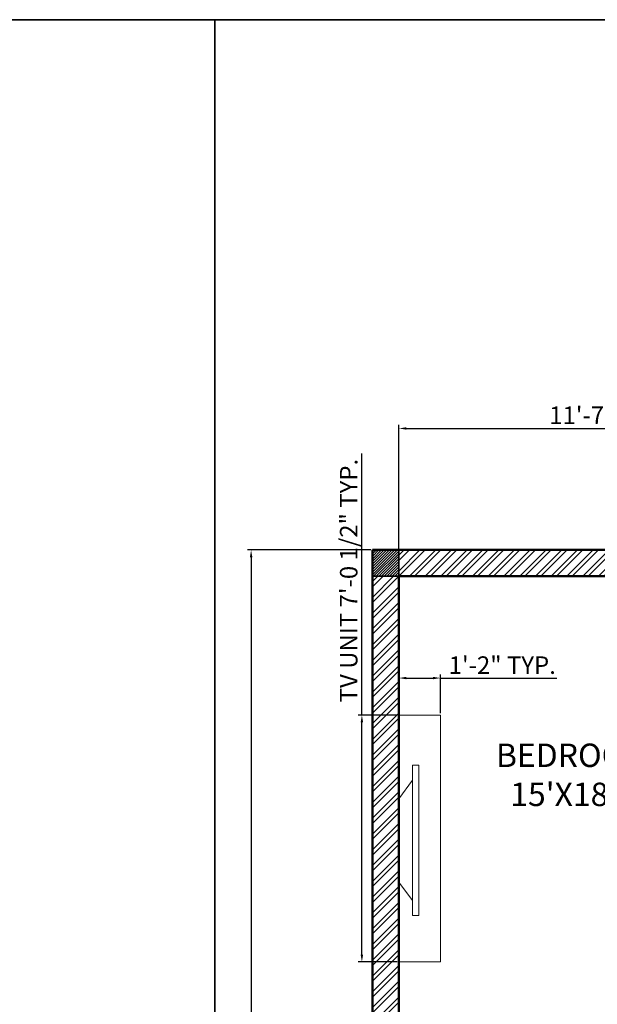
# Model space of a CAD drawing. Units: millimetres. Extents: x 20768 to 23556, y 50760 to 52704.
# Tile 26 of 36: x 21205 to 21403, y 52368 to 52704. Entities that reach past the tile are written whole.
import ezdxf

# ---------------------------------------------------------------- set-up
doc = ezdxf.new("R2010")
doc.units = ezdxf.units.MM
for name, color, linetype, lineweight in [('A-ANNO-TTLB', 7, 'Continuous', 35), ('A-AREA-IDEN', 40, 'Continuous', 18), ('A-FURN', 8, 'Continuous', 18), ('A-WALL', 7, 'Continuous', 50), ('A-WALL-PATT', 8, 'Continuous', 13), ('S-ANNO-DIMS', 2, 'Continuous', 18), ('S-COLS', 20, 'Continuous', 35)]:
    doc.layers.add(name, color=color, linetype=linetype, lineweight=lineweight)
doc.styles.get("Standard").update_dxf_attribs({"font": 'arial.ttf'})
doc.dimstyles.new('ISO-25', dxfattribs={"dimtxt": 6, "dimasz": 2.5, "dimexe": 1.25, "dimexo": 0.625, "dimtad": 1, "dimdec": 0, "dimlunit": 3, "dimtxsty": 'Standard', "dimcen": 2.5, "dimadec": 0, "dimazin": 0, "dimtfac": 1, "dimtdec": 0, "dimtmove": 0, "dimatfit": 3, "dimfxl": 1, "dimarcsym": 0})
pattern_1 = [(45, (-37.4434, 0), (-2.69407684, 2.69407684), []), (45, (-35.6473, 0), (-2.69407684, 2.69407684), [])]

# ---------------------------------------------------------------- blocks, each defined once
blk = doc.blocks.new('tv')
for p, q in [((20989.25, 52437.95), (20993.93, 52444.3)), ((20989.25, 52409.51), (20993.93, 52403.15))]:
    blk.add_line(p, q)
for points in [[(20989.25, 52466.51), (21003.46, 52466.51), (21003.46, 52382.21), (20989.25, 52382.21)], [(20993.93, 52449.42), (20996.05, 52449.42), (20996.05, 52398.03), (20993.93, 52398.03)]]:
    blk.add_lwpolyline(points, close=True)
blk = doc.blocks.new('*D183')
at = {"layer": 'Defpoints', "color": 0, "transparency": 16777216}
for p in [(21322.1, 52466.51), (21334.74, 52466.51), (21334.74, 52382.21)]:
    blk.add_point(p, dxfattribs=at)
at = {"layer": 'S-ANNO-DIMS', "color": 0, "lineweight": -2, "transparency": 16777216}
for p, q in [((21322.1, 52466.51), (21322.1, 52555.89)), ((21334.12, 52466.51), (21320.85, 52466.51)), ((21322.1, 52384.71), (21322.1, 52464.01)), ((21334.12, 52382.21), (21320.85, 52382.21))]:
    blk.add_line(p, q, dxfattribs=at)
at = {"layer": 'S-ANNO-DIMS', "color": 0, "transparency": 16777216}
for points in [[(21321.68, 52464.01), (21322.51, 52464.01), (21322.1, 52466.51)], [(21321.68, 52384.71), (21322.51, 52384.71), (21322.1, 52382.21)]]:
    blk.add_solid(points, dxfattribs=at)
at = {"layer": 'S-ANNO-DIMS', "color": 0, "transparency": 16777216, "insert": (21318.37, 52512.45), "char_height": 6, "attachment_point": 5, "rotation": 90}
blk.add_mtext('TV UNIT 7\'-0 1/2" TYP.', dxfattribs=at)
blk = doc.blocks.new('*D184')
at = {"layer": 'Defpoints', "color": 0, "transparency": 16777216}
for p in [(21348.95, 52479.16), (21334.74, 52466.51), (21348.95, 52466.51)]:
    blk.add_point(p, dxfattribs=at)
at = {"layer": 'S-ANNO-DIMS', "color": 0, "lineweight": -2, "transparency": 16777216}
for p, q in [((21334.74, 52467.14), (21334.74, 52480.41)), ((21348.95, 52467.14), (21348.95, 52480.41)), ((21337.24, 52479.16), (21346.45, 52479.16)), ((21348.95, 52479.16), (21388.71, 52479.16))]:
    blk.add_line(p, q, dxfattribs=at)
at = {"layer": 'S-ANNO-DIMS', "color": 0, "transparency": 16777216}
for points in [[(21337.24, 52479.57), (21337.24, 52478.74), (21334.74, 52479.16)], [(21346.45, 52479.57), (21346.45, 52478.74), (21348.95, 52479.16)]]:
    blk.add_solid(points, dxfattribs=at)
at = {"layer": 'S-ANNO-DIMS', "color": 0, "transparency": 16777216, "insert": (21370.08, 52482.79), "char_height": 6, "attachment_point": 5}
blk.add_mtext('1\'-2" TYP.', dxfattribs=at)
blk = doc.blocks.new('*D211')
at = {"layer": 'Defpoints', "color": 0, "transparency": 16777216}
for p in [(21325.74, 52522.9), (21284.24, 51829.9), (21325.74, 51829.9)]:
    blk.add_point(p, dxfattribs=at)
at = {"layer": 'S-ANNO-DIMS', "color": 0, "lineweight": -2, "transparency": 16777216}
for p, q in [((21325.12, 52522.9), (21282.99, 52522.9)), ((21284.24, 52520.4), (21284.24, 51832.4)), ((21325.12, 51829.9), (21282.99, 51829.9))]:
    blk.add_line(p, q, dxfattribs=at)
at = {"layer": 'S-ANNO-DIMS', "color": 0, "transparency": 16777216}
for points in [[(21283.82, 52520.4), (21284.66, 52520.4), (21284.24, 52522.9)], [(21283.82, 51832.4), (21284.66, 51832.4), (21284.24, 51829.9)]]:
    blk.add_solid(points, dxfattribs=at)
at = {"layer": 'S-ANNO-DIMS', "color": 0, "transparency": 16777216, "insert": (21280.55, 52176.4), "char_height": 6, "attachment_point": 5, "rotation": 90}
blk.add_mtext('57\'-9"', dxfattribs=at)
blk = doc.blocks.new('*D215')
at = {"layer": 'Defpoints', "color": 0, "transparency": 16777216}
for p in [(21474.24, 52564.4), (21334.74, 52329.4), (21474.24, 52329.4)]:
    blk.add_point(p, dxfattribs=at)
at = {"layer": 'S-ANNO-DIMS', "color": 0, "lineweight": -2, "transparency": 16777216}
for p, q in [((21334.74, 52330.02), (21334.74, 52565.65)), ((21337.24, 52564.4), (21471.74, 52564.4)), ((21474.24, 52330.02), (21474.24, 52565.65))]:
    blk.add_line(p, q, dxfattribs=at)
at = {"layer": 'S-ANNO-DIMS', "color": 0, "transparency": 16777216}
for points in [[(21337.24, 52564.81), (21337.24, 52563.98), (21334.74, 52564.4)], [(21471.74, 52564.81), (21471.74, 52563.98), (21474.24, 52564.4)]]:
    blk.add_solid(points, dxfattribs=at)
at = {"layer": 'S-ANNO-DIMS', "color": 0, "transparency": 16777216, "insert": (21404.49, 52568.12), "char_height": 6, "attachment_point": 5}
blk.add_mtext('11\'-7 1/2"', dxfattribs=at)

msp = doc.modelspace()

# ---------------------------------------------------------------- hatches: boundary and pattern name
at = {"layer": 'A-WALL-PATT'}
h = msp.add_hatch(dxfattribs=at)
h.set_pattern_fill('ANSI31', color=256, scale=0.2)
h.set_pattern_definition([(45, (345.4904, 0), (-0.449012806, 0.449012806), [])])
h.paths.add_polyline_path([(21334.74, 52522.9), (21325.74, 52522.9), (21325.74, 52513.9), (21334.74, 52513.9)])
h = msp.add_hatch(dxfattribs=at)
h.set_pattern_fill('ANSI32', color=256, scale=0.4)
h.set_pattern_definition(pattern_1)
h.paths.add_polyline_path([(21550.74, 52522.9), (21334.74, 52522.9), (21334.74, 52513.9), (21550.74, 52513.9)])
h = msp.add_hatch(dxfattribs=at)
h.set_pattern_fill('ANSI32', color=256, scale=0.4)
h.set_pattern_definition(pattern_1)
h.paths.add_polyline_path([(21334.74, 52513.9), (21325.74, 52513.9), (21325.74, 52335.9), (21334.74, 52335.9)])

# ---------------------------------------------------------------- linework, layer by layer
at = {"layer": 'A-ANNO-TTLB'}
msp.add_line((21271.86, 52703.98), (21271.86, 51623.53), dxfattribs=at)
msp.add_lwpolyline([(20768.14, 52703.98), (23555.8, 52703.98), (23555.8, 51623.53), (20768.14, 51623.53)], close=True, dxfattribs=at)
at = {"layer": 'A-WALL'}
for p, q in [((21325.74, 52522.9), (21325.74, 51829.9)), ((21325.74, 52522.9), (21559.74, 52522.9)), ((21334.74, 52513.9), (21334.74, 51829.9)), ((21334.74, 52513.9), (21550.74, 52513.9))]:
    msp.add_line(p, q, dxfattribs=at)
at = {"layer": 'S-COLS'}
msp.add_lwpolyline([(21334.74, 52513.9), (21325.74, 52513.9), (21325.74, 52522.9), (21334.74, 52522.9)], close=True, dxfattribs=at)

# ---------------------------------------------------------------- block references
at = {"layer": 'A-FURN'}
msp.add_blockref('tv', (345.49, 0), dxfattribs=at)

# ---------------------------------------------------------------- texts
at = {"layer": 'A-AREA-IDEN', "insert": (21367.92, 52456.78), "char_height": 8, "attachment_point": 1}
msp.add_mtext_dynamic_manual_height_columns("BEDROOM\\P  15'X18'", width=49.9521, gutter_width=12.5, heights=[0], dxfattribs=at)

# ---------------------------------------------------------------- dimensions: what is measured, and where the dimension line sits
at = {"layer": 'S-ANNO-DIMS'}
dim = msp.add_linear_dim(base=(21474.24, 52564.4), p1=(21334.74, 52329.4), p2=(21474.24, 52329.4), dimstyle='ISO-25', override={"dimdec": 1, "dimlfac": 1, "dimrnd": 0, "dimzin": 1, "dimdsep": 46, "dimlunit": 4, "dimfrac": 2}, dxfattribs=at)
dim.commit()
dim.dimension.update_dxf_attribs({"geometry": '*D215', "text_midpoint": (21404.49, 52568.12)})
dim = msp.add_linear_dim(base=(21322.1, 52466.51), p1=(21334.74, 52382.21), p2=(21334.74, 52466.51), angle=90, text='TV UNIT <> TYP.', dimstyle='ISO-25', override={"dimdec": 1, "dimrnd": 0, "dimzin": 1, "dimlunit": 4, "dimfrac": 2}, dxfattribs=at)
dim.commit()
dim.dimension.update_dxf_attribs({"geometry": '*D183', "text_midpoint": (21318.37, 52512.45)})
dim = msp.add_linear_dim(base=(21284.24, 51829.9), p1=(21325.74, 52522.9), p2=(21325.74, 51829.9), angle=90, dimstyle='ISO-25', override={"dimdec": 1, "dimlfac": 1, "dimrnd": 0, "dimzin": 1, "dimdsep": 46, "dimlunit": 4, "dimfrac": 2}, dxfattribs=at)
dim.commit()
dim.dimension.update_dxf_attribs({"geometry": '*D211', "text_midpoint": (21280.55, 52176.4)})
dim = msp.add_linear_dim(base=(21348.95, 52479.16), p1=(21334.74, 52466.51), p2=(21348.95, 52466.51), text='<> TYP.', dimstyle='ISO-25', override={"dimdec": 1, "dimrnd": 0, "dimzin": 1, "dimlunit": 4, "dimfrac": 2}, dxfattribs=at)
dim.commit()
dim.dimension.update_dxf_attribs({"geometry": '*D184', "text_midpoint": (21370.08, 52482.79)})

doc.saveas('drawing.dxf')
